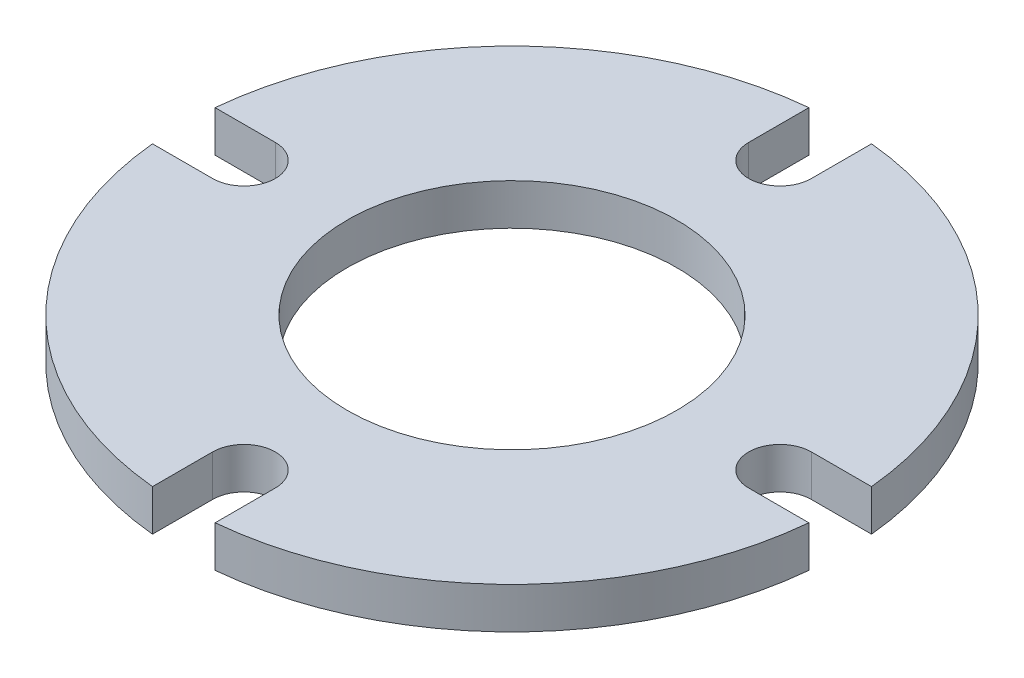
from build123d import *

# Parameters (mm, degrees)
DISK_PROFILE_SKETCH_R       = 50
SLOTTED_DISK_200X12_5_DEPTH = 6.25


with BuildPart() as part:
    # Disk Profile Sketch → Slotted Disk Ø200x12.5 (new, symmetric)
    with BuildSketch(Plane(origin=(0, 0, 0), x_dir=(1, 0, 0), z_dir=(0, 1, 0))):
        with BuildLine():
            Line((-9.5, 81.3), (-9.5, 99.547727247))
            ThreePointArc((-9.5, 99.547727247), (-70.710678119, 70.710678119), (-99.547727247, 9.5))
            Line((-99.547727247, 9.5), (-81.3, 9.5))
            ThreePointArc((-81.3, 9.5), (-71.8, 0), (-81.3, -9.5))
            Line((-81.3, -9.5), (-99.547727247, -9.5))
            ThreePointArc((-99.547727247, -9.5), (-70.710678119, -70.710678119), (-9.5, -99.547727247))
            Line((-9.5, -99.547727247), (-9.5, -81.3))
            ThreePointArc((-9.5, -81.3), (0, -71.8), (9.5, -81.3))
            Line((9.5, -81.3), (9.5, -99.547727247))
            ThreePointArc((9.5, -99.547727247), (70.710678119, -70.710678119), (99.547727247, -9.5))
            Line((99.547727247, -9.5), (81.3, -9.5))
            ThreePointArc((81.3, -9.5), (71.8, 0), (81.3, 9.5))
            Line((81.3, 9.5), (99.547727247, 9.5))
            ThreePointArc((99.547727247, 9.5), (70.710678119, 70.710678119), (9.5, 99.547727247))
            Line((9.5, 99.547727247), (9.5, 81.3))
            ThreePointArc((9.5, 81.3), (0, 71.8), (-9.5, 81.3))
        make_face()
        with Locations(Location((0, 0, 0), (0, 0, 270))):
            Circle(DISK_PROFILE_SKETCH_R, mode=Mode.SUBTRACT)
    extrude(amount=SLOTTED_DISK_200X12_5_DEPTH, both=True)


solid = part.part
